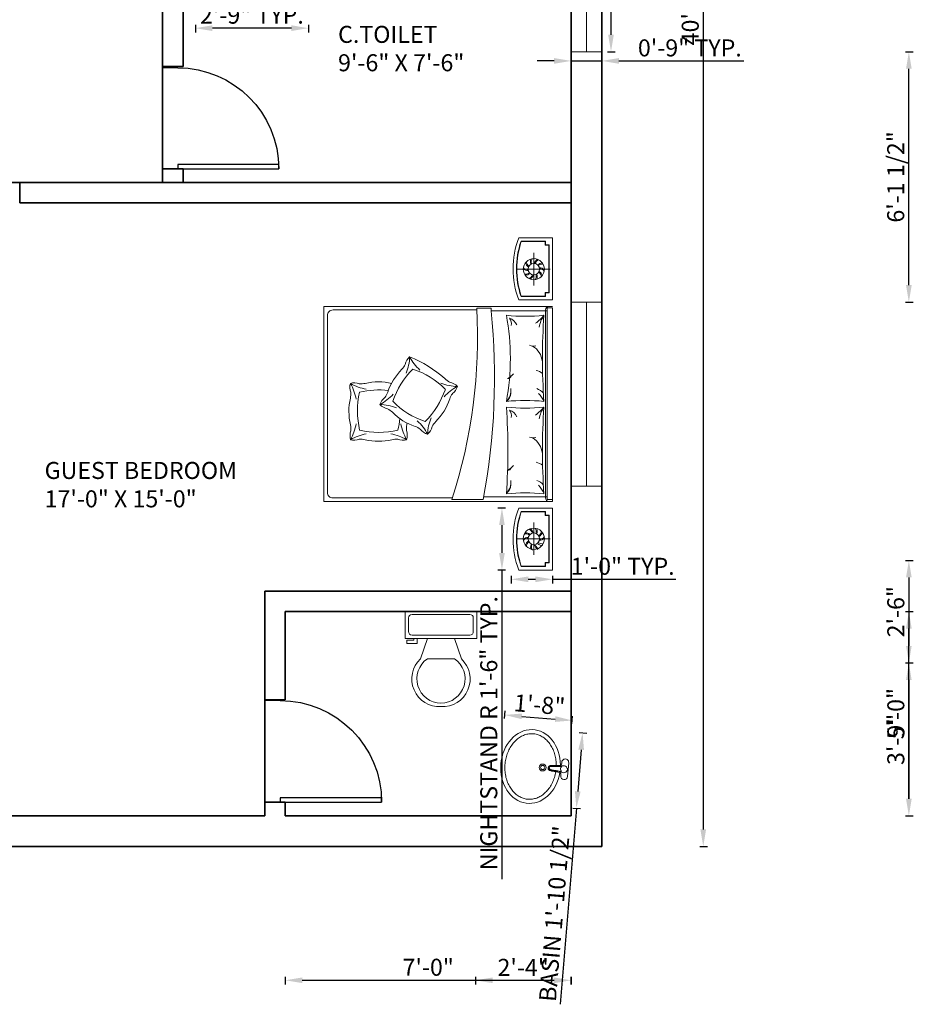
# Model space of a CAD drawing. Units: inches. Extents: x -48 to 817, y -530 to 78.
# Tile 5 of 7: x 551 to 817, y -515 to -225. Entities that reach past the tile are written whole.
import ezdxf

# ---------------------------------------------------------------- set-up
doc = ezdxf.new("R2010")
doc.units = ezdxf.units.IN
for name, color, linetype, lineweight in [('A-ANNO-DIMS', 2, 'Continuous', 18), ('A-AREA-IDEN', 7, 'Continuous', 18), ('A-DOOR', 3, 'Continuous', 25), ('A-FLOR-FIXT', 9, 'Continuous', 18), ('A-GLAZ', 4, 'Continuous', 18), ('A-WALL', 7, 'Continuous', 35), ('furn', 8, 'Continuous', 18)]:
    doc.layers.add(name, color=color, linetype=linetype, lineweight=lineweight)
doc.styles.get("Standard").update_dxf_attribs({"font": 'arial.ttf'})
doc.dimstyles.new('ISO-25', dxfattribs={"dimtxt": 5, "dimasz": 5, "dimexe": 1.25, "dimexo": 0.625, "dimtad": 1, "dimlunit": 3, "dimtxsty": 'Standard', "dimcen": 2.5, "dimadec": 0, "dimazin": 0, "dimtfac": 1, "dimtmove": 0, "dimatfit": 3, "dimfxl": 1, "dimfxlon": 1, "dimarcsym": 0})

# ---------------------------------------------------------------- blocks, each defined once
blk = doc.blocks.new('*U4')
for p, q in [((9.5, -6), (9.5, -2)), ((-10, -8.5), (-8, -8.5)), ((-10, -9.5), (-10, -8.5)), ((-8, -8.5), (-8, -8)), ((-7, -8), (-7, -9.5)), ((-4, -8), (-6, -14)), ((4, -8), (6, -14)), ((-7, -9.5), (-10, -9.5)), ((4, -14), (-4, -14))]:
    blk.add_line(p, q)
blk.add_lwpolyline([(10.5, -8), (10.5, 0), (-10.5, 0), (-10.5, -8)], close=True)
for points in [[(-9.5, -2), (-9.5, -6)], [(8.5, -1), (-8.5, -1)], [(-8.5, -7), (8.5, -7)]]:
    blk.add_lwpolyline(points)
for centre, radius, start, end in [((-8.625, -1.875), 0.8839, 81.8699, 188.1301), ((8.625, -1.875), 0.8839, 351.8699, 98.1301), ((-8.625, -6.125), 0.8839, 171.869898, 278.1301), ((8.625, -6.125), 0.8839, 261.8699, 8.1301), ((-0.4772, -19.9188), 8.0953, 133.01722, 273.38), ((0.0374, -19.8731), 7.127, 124.50543, 269.7), ((-0.0373, -19.8731), 7.127, 270.3, 55.4946), ((0.4773, -19.9188), 8.0953, 266.62, 46.9828)]:
    blk.add_arc(centre, radius, start, end)
blk = doc.blocks.new('*U2')
for p, q in [((0, 0), (0, -6)), ((40, 0), (40, -6))]:
    blk.add_line(p, q)
blk.add_lwpolyline([(0, 0), (0, 40), (1.75, 40), (1.75, 0)], close=True)
blk.add_arc((0, 0), 40, 0, 90)
blk = doc.blocks.new('A$C359865C9')
for p, q in [((0.26, 0.5858), (0.38, 0.5858)), ((0.26, 0.5258), (0.272, 0.5258)), ((0.368, 0.5258), (0.3809, 0.5258))]:
    blk.add_line(p, q)
for radius in [0.03, 0.018]:
    blk.add_circle((0.3201, 0.3632), radius)
for centre, radius, start, end in [((0.26, 0.5558), 0.03, 90.00613, 270.00613), ((0.272, 0.5078), 0.018, 0.00613, 90.00613), ((0.32, 0.5495), 0.03, 348.15369, 191.84631), ((0.32, 0.5495), 0.03, 222.45226, 317.54774), ((0.368, 0.5078), 0.018, 90.00613, 180.00613), ((0.38, 0.5558), 0.03, 270.00613, 89.98161), ((0.3201, 0.4358), 0.024, 180.00613, 0.00613), ((0.3201, 0.4358), 0.0204, 180.00613, 0.00613), ((0.3201, 0.4358), 0.0144, 180.00613, 0.00613)]:
    blk.add_arc(centre, radius, start, end)
at = {"ltscale": 100, "extrusion": (0, 0, -1)}
blk.add_ellipse((0.3201, 0.258), major_axis=(0.3216, 0), ratio=0.80597, start_param=-1.471508, end_param=4.612925, dxfattribs=at)
at = {"extrusion": (0, 0, -1)}
blk.add_ellipse((0.3199, 0.5826), major_axis=(-0.00812, 0), ratio=0.392595, dxfattribs=at)
for points, knots in [([(0.2907, 0.5434), (0.2946, 0.498), (0.2952, 0.4908), (0.2965, 0.4761), (0.2971, 0.4686), (0.2983, 0.4536), (0.2989, 0.4461), (0.2995, 0.4378), (0.2996, 0.4369), (0.2996, 0.4361)], [2.511178, 2.511178, 2.511178, 2.511178, 20.495008, 20.495008, 39.297594, 39.297594, 58.10018, 58.10018, 60.208758, 60.208758, 60.208758, 60.208758]), ([(0.2979, 0.5293), (0.298, 0.528), (0.2981, 0.5267), (0.2988, 0.5184), (0.2993, 0.5127), (0.3005, 0.4986), (0.301, 0.4933), (0.3014, 0.4884), (0.3015, 0.4875), (0.3017, 0.4857), (0.3017, 0.485), (0.3019, 0.4827), (0.3021, 0.4812), (0.3026, 0.4756), (0.3029, 0.4716), (0.3037, 0.4621), (0.3041, 0.4568), (0.3049, 0.4464), (0.3053, 0.4415), (0.3056, 0.4365)], [4.643985, 4.643985, 4.643985, 4.643985, 5.282102, 5.282102, 8.976667, 8.976667, 16.365798, 16.365798, 18.536065, 18.536065, 20.434607, 20.434607, 24.231692, 24.231692, 34.371999, 34.371999, 47.807513, 47.807513, 60.208758, 60.208758, 60.208758, 60.208758]), ([(0.3422, 0.5293), (0.3421, 0.528), (0.342, 0.5267), (0.3412, 0.5184), (0.3408, 0.5127), (0.3395, 0.4986), (0.3391, 0.4933), (0.3387, 0.4884), (0.3386, 0.4875), (0.3384, 0.4857), (0.3383, 0.485), (0.3381, 0.4827), (0.338, 0.4812), (0.3375, 0.4756), (0.3372, 0.4716), (0.3364, 0.4621), (0.336, 0.4568), (0.3352, 0.4464), (0.3348, 0.4415), (0.3345, 0.4365)], [4.643985, 4.643985, 4.643985, 4.643985, 5.282102, 5.282102, 8.976667, 8.976667, 16.365798, 16.365798, 18.536065, 18.536065, 20.434607, 20.434607, 24.231692, 24.231692, 34.371999, 34.371999, 47.807513, 47.807513, 60.208758, 60.208758, 60.208758, 60.208758]), ([(0.3494, 0.5434), (0.3455, 0.498), (0.3449, 0.4908), (0.3436, 0.4761), (0.343, 0.4686), (0.3418, 0.4536), (0.3412, 0.4461), (0.3406, 0.4378), (0.3405, 0.4369), (0.3404, 0.4361)], [2.511178, 2.511178, 2.511178, 2.511178, 20.495008, 20.495008, 39.297594, 39.297594, 58.10018, 58.10018, 60.208758, 60.208758, 60.208758, 60.208758]), ([(0.3475, 0.4801), (0.3477, 0.4801), (0.3479, 0.4801), (0.3648, 0.4788), (0.3813, 0.4763), (0.4136, 0.4692), (0.4293, 0.4645), (0.4593, 0.4531), (0.4737, 0.4464), (0.5006, 0.4312), (0.5131, 0.4227), (0.5361, 0.4042), (0.5465, 0.3942), (0.5649, 0.3732), (0.5729, 0.3622), (0.5864, 0.3393), (0.5918, 0.3275), (0.6, 0.3036), (0.6029, 0.2914), (0.6059, 0.2669), (0.6061, 0.2545), (0.6039, 0.2301), (0.6015, 0.218), (0.5941, 0.1942), (0.5892, 0.1825), (0.5768, 0.1597), (0.5693, 0.1486), (0.552, 0.1275), (0.5422, 0.1174), (0.5203, 0.0986), (0.5083, 0.0899), (0.4825, 0.0741), (0.4686, 0.0671), (0.4396, 0.0549), (0.4243, 0.0498), (0.3929, 0.0418), (0.3767, 0.0388), (0.3439, 0.0352), (0.3273, 0.0344), (0.2942, 0.0353), (0.2776, 0.0369), (0.2452, 0.0422), (0.2293, 0.046), (0.1987, 0.0556), (0.1839, 0.0615), (0.156, 0.0751), (0.1428, 0.0828), (0.1184, 0.0997), (0.1071, 0.109), (0.0869, 0.1288), (0.078, 0.1393), (0.0625, 0.1611), (0.0559, 0.1725), (0.0454, 0.1957), (0.0415, 0.2076), (0.036, 0.2317), (0.0346, 0.2438), (0.0345, 0.2566), (0.0345, 0.2573), (0.0345, 0.258), (0.0345, 0.2664), (0.0351, 0.2749), (0.0382, 0.2956), (0.0413, 0.3078), (0.0502, 0.3317), (0.0559, 0.3434), (0.0699, 0.3661), (0.0782, 0.377), (0.0972, 0.3978), (0.1079, 0.4076), (0.1313, 0.4257), (0.1441, 0.434), (0.1714, 0.4488), (0.186, 0.4553), (0.2163, 0.4662), (0.2321, 0.4706), (0.2628, 0.4769), (0.2776, 0.479), (0.2925, 0.4801)], [1.664851, 1.664851, 1.664851, 1.664851, 1.666804, 1.666804, 1.838807, 1.838807, 2.01081, 2.01081, 2.182814, 2.182814, 2.354817, 2.354817, 2.52682, 2.52682, 2.698824, 2.698824, 2.870827, 2.870827, 3.04283, 3.04283, 3.214834, 3.214834, 3.384783, 3.384783, 3.554732, 3.554732, 3.724681, 3.724681, 3.89463, 3.89463, 4.064578, 4.064578, 4.234527, 4.234527, 4.404476, 4.404476, 4.574425, 4.574425, 4.744374, 4.744374, 4.914323, 4.914323, 5.084272, 5.084272, 5.254221, 5.254221, 5.42417, 5.42417, 5.594119, 5.594119, 5.764068, 5.764068, 5.934016, 5.934016, 6.103965, 6.103965, 6.273914, 6.273914, 6.283185, 6.283185, 6.283185, 6.401959, 6.401959, 6.573962, 6.573962, 6.745965, 6.745965, 6.917969, 6.917969, 7.089972, 7.089972, 7.261975, 7.261975, 7.433979, 7.433979, 7.605982, 7.605982, 7.759676, 7.759676, 7.759676, 7.759676]), ([(0.29, 0.5078), (0.2913, 0.4937), (0.2935, 0.4697), (0.2953, 0.4457), (0.2961, 0.4358)], [0, 0, 0, 0, 35.358253, 60.208758, 60.208758, 60.208758, 60.208758]), ([(0.35, 0.5078), (0.3487, 0.4937), (0.3466, 0.4697), (0.3448, 0.4457), (0.344, 0.4358)], [0, 0, 0, 0, 35.358253, 60.208758, 60.208758, 60.208758, 60.208758])]:
    blk.add_open_spline(points, degree=3, knots=knots)
blk = doc.blocks.new('*D10')
at = {"layer": 'A-ANNO-DIMS', "color": 0, "lineweight": -2, "transparency": 16777216}
for p, q in [((751.22, 11.72), (753.47, 11.72)), ((752.22, 6.72), (752.22, -463.28)), ((751.22, -468.28), (753.47, -468.28))]:
    blk.add_line(p, q, dxfattribs=at)
at = {"layer": 'A-ANNO-DIMS', "color": 0, "transparency": 16777216}
for points in [[(751.39, 6.72), (753.06, 6.72), (752.22, 11.72)], [(751.39, -463.28), (753.06, -463.28), (752.22, -468.28)]]:
    blk.add_solid(points, dxfattribs=at)
at = {"layer": 'Defpoints', "color": 0, "transparency": 16777216}
for p in [(729.44, 11.72), (722.43, -468.28), (752.22, -468.28)]:
    blk.add_point(p, dxfattribs=at)
at = {"layer": 'A-ANNO-DIMS', "color": 0, "transparency": 16777216, "insert": (749.05, -228.28), "char_height": 5, "attachment_point": 5, "rotation": 90}
blk.add_mtext("40'", dxfattribs=at)
blk = doc.blocks.new('BED-DOUBLE')
for p, q in [((0.99, 65.08), (56.21, 65.08)), ((1.28, 65.57), (1.28, 49.06)), ((55.89, 65.57), (55.89, 46.91))]:
    blk.add_line(p, q)
for points in [[(0, 67.12), (0, 0), (57.2, 0), (57.2, 67.12)], [(56.67, 67.12), (56.67, 65.57), (0.33, 65.57), (0.33, 67.12), (57.2, 67.12)]]:
    blk.add_lwpolyline(points)
for points in [[(2.54, 53.57, 0.058596), (2.54, 64.62, 0.036889), (27.85, 64.62, 0.052163), (27.85, 53.57, 0.093111)], [(29.5, 53.57, 0.058596), (29.5, 64.62, 0.036648), (54.99, 64.62, 0.052163), (54.99, 53.57, 0.036967)], [(0.5, 49.06), (1.28, 49.06, -0.072944), (56.67, 46.75), (56.67, 37.58, 0.092568), (0.5, 44.85)]]:
    blk.add_lwpolyline(points, format="xyb", close=True)
for points in [[(0.99, 44.88), (0.99, 2.65, 0.414214), (2.65, 0.99), (54.56, 0.99, 0.414214), (56.21, 2.65), (56.21, 37.74)], [(22.46, 34.35, 0.091296), (23.47, 39.19, 0.091296), (26.52, 35.29, 0.091296)], [(18.37, 26.07, 0.111006), (27.81, 20.2, 0.119549), (33.77, 29.75, 0.107813), (24.35, 35.65)], [(24.3, 35.64, 0.121865), (18.37, 26.07, 0.121865)], [(28.76, 16.41, 0.159461), (30.04, 18.69, -0.076283), (31.05, 20.1, 0.115075), (35.2, 26.76, -0.076283), (36.02, 28.3, 0.159461), (37.5, 30.45)], [(32.66, 31.47, 0.091296), (37.5, 30.45, 0.091296), (33.59, 27.41, 0.091296)], [(19.57, 24.14, 0.091296), (14.72, 25.16, 0.091296), (18.63, 28.19, 0.091296)], [(34.44, 22.59, 0.091296), (39.09, 24.28, 0.091296), (37.38, 19.64, 0.091296)], [(39.09, 7.75, 0.159461), (38.98, 10.35, -0.076283), (39.09, 12.09, 0.115075), (39.09, 19.94, -0.076283), (38.98, 21.68, 0.159461), (39.09, 24.28)], [(25.17, 10.45, 0.111006), (36.29, 10.46, 0.119549), (36.29, 21.72, 0.033212), (32.87, 22.24)], [(29.76, 21.26, 0.091296), (28.76, 16.41, 0.091296), (25.71, 20.31)], [(27.21, 9.44, 0.091296), (22.56, 7.75, 0.091296), (24.27, 12.39, 0.091296)], [(37.38, 12.39, 0.091296), (39.09, 7.75, 0.091296), (34.44, 9.44)]]:
    blk.add_lwpolyline(points, format="xyb")
for centre, radius, start, end in [((0.99, 66.07), 0.992, 180, 270), ((8.41, 73.86), 10.95, 237.5379, 257.5233), ((-5.75, 54.29), 13.24, 36.4935, 51.2792), ((16.81, 58.07), 6.13, 96.6849, 148.3182), ((23.01, 61.56), 4.3, 141.8174, 169.8987), ((28.45, 60.95), 4.63, 130.5354, 160.3558), ((31.33, 57.05), 8.33, 114.6457, 134.1585), ((21.22, 54.29), 13.24, 36.4935, 51.2792), ((35.38, 73.86), 10.95, 237.5379, 257.5233), ((43.78, 58.07), 6.13, 96.6849, 148.3182), ((49.97, 61.56), 4.3, 141.8174, 169.8987), ((55.41, 60.95), 4.63, 130.5354, 160.3558), ((58.29, 57.05), 8.33, 114.6457, 134.1585), ((56.21, 66.07), 0.992, 270, 0), ((8.86, 61.48), 2.75, 335.8927, 16.1192), ((35.82, 61.48), 2.75, 335.8927, 16.1192), ((6.89, 53.32), 3.67, 114.2916, 160.9896), ((4.98, 52.55), 2.51, 76.4823, 128.5563), ((9.99, 45.89), 13.8, 36.2085, 45.0849), ((20.2, 54.04), 0.927, 353.7543, 77.2187), ((33.85, 53.32), 3.67, 114.2916, 160.9896), ((31.95, 52.55), 2.51, 76.4823, 128.5563), ((36.95, 45.89), 13.8, 36.2085, 45.0849), ((47.16, 54.04), 0.927, 353.7543, 77.2187), ((24.63, 50.41), 4.52, 44.406, 96.8342), ((25.47, 51.99), 2.86, 33.6349, 90.8456), ((51.59, 50.41), 4.52, 44.406, 96.8342), ((52.44, 51.99), 2.86, 33.6349, 90.8456), ((26.3, 36.1), 4.19, 132.4658, 168.7065), ((22.36, 35.3), 4.04, 37.2937, 74.0973), ((29.01, 42.35), 5.74, 233.2983, 250.7472), ((48.24, 11.46), 36.21, 138.3818, 157.7644), ((17.07, 39.52), 5.74, 315.5854, 333.0343), ((21.6, 20.56), 17.28, 45.1307, 71.3884), ((37.79, 36.92), 5.74, 225.7718, 243.2208), ((34.51, 27.99), 3.87, 39.4726, 79.6505), ((17.81, 28), 4.19, 222.6522, 258.8929), ((14.41, 18.76), 5.74, 45.7718, 63.2208), ((30.83, 7.48), 17.28, 77.0576, 78.7033), ((35.92, 29.93), 5.74, 257.6988, 275.1477), ((37.86, 20.61), 3.87, 71.3996, 111.5774), ((30.61, 35.12), 17.28, 225.1307, 251.3884), ((39.38, 16.01), 17.28, 166.8711, 193.1289), ((47.91, 16.13), 23.44, 173.1956, 194.0284), ((23.2, 13.33), 5.74, 53.2983, 70.7472), ((30.37, 20.93), 4.79, 218.7754, 250.3571), ((16.95, 10.85), 5.74, 355.0387, 12.4877), ((26.6, 8.88), 4.19, 159.3666, 195.6073), ((23.67, 11.79), 4.19, 254.5791, 290.8198), ((25.68, 2.15), 5.74, 77.6988, 95.1477), ((30.77, 24.6), 17.28, 257.0576, 283.3153), ((36.01, 2.19), 5.74, 85.2252, 102.6741), ((38.07, 12.43), 4.79, 250.7023, 282.284)]:
    blk.add_arc(centre, radius, start, end)
blk = doc.blocks.new('NIGHTSTAND-WITH-LAMP-L')
for p, q in [((9.19, 1.33), (9.19, 10.86)), ((4.42, 6.1), (13.95, 6.1))]:
    blk.add_line(p, q)
blk.add_lwpolyline([(0, 1.65), (0, 11.57), (18.19, 11.57), (18.19, 1.65, -0.181818)], format="xyb", close=True)
for points in [[(2.08, 10.58), (2.08, 9.49), (0.99, 9.49)], [(2.18, 10.58), (2.18, 9.39), (0.99, 9.39)], [(2.08, 10.58), (16.1, 10.58)], [(2.08, 10.48), (16.1, 10.48)], [(16, 10.58), (16, 9.39), (17.19, 9.39)], [(16.1, 10.58), (16.1, 9.49), (17.19, 9.49)]]:
    blk.add_lwpolyline(points)
for points in [[(17.19, 9.49), (17.19, 2.35, -0.167087), (0.99, 2.35), (0.99, 9.49)], [(17.09, 9.49), (17.09, 2.42, -0.165559), (1.09, 2.42), (1.09, 9.49)]]:
    blk.add_lwpolyline(points, format="xyb")
for radius in [3.11, 1.69]:
    blk.add_circle((9.19, 6.1), radius)
for centre, radius, start, end in [((9.46, 8.43), 2, 172.17, 218.4897), ((9.27, 8.39), 1.53, 160.3002, 220.538), ((10.78, 7.82), 2, 136.17, 182.4897), ((10.6, 7.9), 1.53, 124.3002, 184.538), ((8.04, 8.15), 2, 208.17, 254.4897), ((7.91, 8), 1.53, 196.3002, 256.538), ((11.49, 6.56), 2, 100.17, 146.4897), ((11.39, 6.73), 1.53, 88.3002, 148.538), ((11.32, 5.11), 2, 64.17, 110.4897), ((11.34, 5.31), 1.53, 52.3002, 112.538), ((10.33, 4.05), 2, 28.17, 74.4897), ((7.03, 6.88), 1.53, 232.3002, 292.538), ((7.05, 7.08), 2, 244.17, 290.4897), ((6.98, 5.47), 1.53, 268.3002, 328.538), ((6.88, 5.64), 2, 280.17, 326.4897), ((7.78, 4.29), 1.53, 304.3002, 4.538), ((7.59, 4.37), 2, 316.17, 2.4897), ((9.11, 3.81), 1.53, 340.3002, 40.538), ((8.91, 3.76), 2, 352.17, 38.4897), ((10.47, 4.2), 1.53, 16.3002, 76.538)]:
    blk.add_arc(centre, radius, start, end)
blk = doc.blocks.new('NIGHTSTAND-WITH-LAMP-R')
for p, q in [((9, 1.32), (9, 10.86)), ((13.77, 6.09), (4.23, 6.09))]:
    blk.add_line(p, q)
blk.add_lwpolyline([(18.19, 1.65), (18.19, 11.57), (0, 11.57), (0, 1.65, 0.181818)], format="xyb", close=True)
for points in [[(2.08, 10.58), (2.08, 9.49), (0.99, 9.49)], [(2.18, 10.58), (2.18, 9.39), (0.99, 9.39)], [(16.1, 10.58), (2.08, 10.58)], [(16.1, 10.48), (2.08, 10.48)], [(16, 10.58), (16, 9.39), (17.19, 9.39)], [(16.1, 10.58), (16.1, 9.49), (17.19, 9.49)]]:
    blk.add_lwpolyline(points)
for points in [[(0.99, 9.49), (0.99, 2.35, 0.167087), (17.19, 2.35), (17.19, 9.49)], [(1.09, 9.49), (1.09, 2.42, 0.165559), (17.09, 2.42), (17.09, 9.49)]]:
    blk.add_lwpolyline(points, format="xyb")
for radius in [3.11, 1.69]:
    blk.add_circle((9, 6.09), radius)
for centre, radius, start, end in [((7.59, 7.9), 1.53, 355.462, 55.6998), ((7.4, 7.82), 2, 357.5103, 43.83), ((8.92, 8.38), 1.53, 319.462, 19.6998), ((8.95, 8.51), 2, 321.5103, 7.83), ((6.85, 5.31), 1.53, 67.462, 127.6998), ((6.87, 5.11), 2, 69.5103, 115.83), ((7.85, 4.04), 2, 105.5103, 151.83), ((6.8, 6.72), 1.53, 31.462, 91.6998), ((6.69, 6.55), 2, 33.5103, 79.83), ((10.51, 8.08), 1.53, 283.462, 343.6998), ((10.37, 8.23), 2, 285.5103, 331.83), ((7.72, 4.19), 1.53, 103.462, 163.6998), ((9.27, 3.76), 2, 141.5103, 187.83), ((9.08, 3.8), 1.53, 139.462, 199.6998), ((10.59, 4.37), 2, 177.5103, 223.83), ((10.41, 4.29), 1.53, 175.462, 235.6998), ((11.3, 5.63), 2, 213.5103, 259.83), ((11.2, 5.46), 1.53, 211.462, 271.6998), ((11.36, 7.16), 2, 249.5103, 295.83), ((11.38, 6.96), 1.53, 247.462, 307.6998)]:
    blk.add_arc(centre, radius, start, end)
blk = doc.blocks.new('WIN-54IN')
blk.add_line((4.5, 54), (4.5, 0))
blk.add_lwpolyline([(9, 54), (0, 54), (0, 0), (9, 0)], close=True)
blk = doc.blocks.new('WIN-18IN')
blk.add_line((4.5, 18), (4.5, 0))
blk.add_lwpolyline([(0, 18), (9, 18), (9, 0), (0, 0)], close=True)
blk = doc.blocks.new('*D24')
at = {"layer": 'A-ANNO-DIMS', "color": 0, "lineweight": -2, "transparency": 16777216}
for p, q in [((725.13, -216.89), (725.13, -147.37)), ((724.13, -216.89), (726.38, -216.89)), ((725.13, -229.89), (725.13, -221.89)), ((724.13, -234.89), (726.38, -234.89))]:
    blk.add_line(p, q, dxfattribs=at)
at = {"layer": 'A-ANNO-DIMS', "color": 0, "transparency": 16777216}
for points in [[(724.29, -221.89), (725.96, -221.89), (725.13, -216.89)], [(724.29, -229.89), (725.96, -229.89), (725.13, -234.89)]]:
    blk.add_solid(points, dxfattribs=at)
at = {"layer": 'Defpoints', "color": 0, "transparency": 16777216}
for p in [(722.43, -216.89), (725.13, -216.89), (722.43, -234.89)]:
    blk.add_point(p, dxfattribs=at)
at = {"layer": 'A-ANNO-DIMS', "color": 0, "transparency": 16777216, "insert": (721.92, -179.63), "char_height": 5, "attachment_point": 5, "rotation": 90}
blk.add_mtext('WINDOW 1\'-6" TYP.', dxfattribs=at)
blk = doc.blocks.new('*D25')
at = {"layer": 'A-ANNO-DIMS', "color": 0, "lineweight": -2, "transparency": 16777216}
for p, q in [((713.43, -236.59), (713.43, -238.84)), ((722.43, -236.59), (722.43, -238.84)), ((708.43, -237.59), (703.43, -237.59)), ((713.43, -237.59), (722.43, -237.59)), ((727.43, -237.59), (764.15, -237.59))]:
    blk.add_line(p, q, dxfattribs=at)
at = {"layer": 'A-ANNO-DIMS', "color": 0, "transparency": 16777216}
for points in [[(708.43, -236.75), (708.43, -238.42), (713.43, -237.59)], [(727.43, -236.75), (727.43, -238.42), (722.43, -237.59)]]:
    blk.add_solid(points, dxfattribs=at)
at = {"layer": 'Defpoints', "color": 0, "transparency": 16777216}
for p in [(713.43, -234.89), (722.43, -234.89), (722.43, -237.59)]:
    blk.add_point(p, dxfattribs=at)
at = {"layer": 'A-ANNO-DIMS', "color": 0, "transparency": 16777216, "insert": (748.29, -234.41), "char_height": 5, "attachment_point": 5}
blk.add_mtext('0\'-9" TYP.', dxfattribs=at)
blk = doc.blocks.new('*D29')
at = {"layer": 'A-ANNO-DIMS', "color": 0, "lineweight": -2, "transparency": 16777216}
for p, q in [((603.04, -226.97), (603.04, -229.22)), ((631.24, -227.97), (608.04, -227.97)), ((636.24, -226.97), (636.24, -229.22))]:
    blk.add_line(p, q, dxfattribs=at)
at = {"layer": 'A-ANNO-DIMS', "color": 0, "transparency": 16777216}
for points in [[(608.04, -227.13), (608.04, -228.8), (603.04, -227.97)], [(631.24, -227.13), (631.24, -228.8), (636.24, -227.97)]]:
    blk.add_solid(points, dxfattribs=at)
at = {"layer": 'Defpoints', "color": 0, "transparency": 16777216}
for p in [(603.04, -222.37), (636.24, -222.37), (603.04, -227.97)]:
    blk.add_point(p, dxfattribs=at)
at = {"layer": 'A-ANNO-DIMS', "color": 0, "transparency": 16777216, "insert": (619.64, -224.79), "char_height": 5, "attachment_point": 5}
blk.add_mtext('2\'-9" TYP.', dxfattribs=at)
blk = doc.blocks.new('*D30')
at = {"layer": 'A-ANNO-DIMS', "color": 0, "lineweight": -2, "transparency": 16777216}
for p, q in [((715.77, -434.81), (718.01, -434.99)), ((716.36, -439.87), (715.36, -452.1)), ((714.95, -457.08), (710.23, -514.64)), ((713.95, -457), (716.19, -457.18))]:
    blk.add_line(p, q, dxfattribs=at)
at = {"layer": 'A-ANNO-DIMS', "color": 0, "transparency": 16777216}
for points in [[(715.53, -439.81), (717.19, -439.94), (716.77, -434.89)], [(714.53, -452.03), (716.19, -452.17), (714.95, -457.08)]]:
    blk.add_solid(points, dxfattribs=at)
at = {"layer": 'Defpoints', "color": 0, "transparency": 16777216}
for p in [(713.44, -434.62), (711.62, -456.81), (714.95, -457.08)]:
    blk.add_point(p, dxfattribs=at)
at = {"layer": 'A-ANNO-DIMS', "color": 0, "transparency": 16777216, "insert": (709.19, -488.09), "char_height": 5, "attachment_point": 5, "rotation": 85.3161}
blk.add_mtext('BASIN 1\'-10 1/2"', dxfattribs=at)
blk = doc.blocks.new('*D31')
at = {"layer": 'A-ANNO-DIMS', "color": 0, "lineweight": -2, "transparency": 16777216}
for p, q in [((693.87, -430.67), (694.06, -428.42)), ((698.94, -430.08), (708.73, -430.88)), ((713.63, -432.29), (713.81, -430.04))]:
    blk.add_line(p, q, dxfattribs=at)
at = {"layer": 'A-ANNO-DIMS', "color": 0, "transparency": 16777216}
for points in [[(699.01, -429.25), (698.87, -430.91), (693.95, -429.67)], [(708.79, -430.05), (708.66, -431.71), (713.71, -431.29)]]:
    blk.add_solid(points, dxfattribs=at)
at = {"layer": 'Defpoints', "color": 0, "transparency": 16777216}
for p in [(693.68, -433), (713.71, -431.29), (713.44, -434.62)]:
    blk.add_point(p, dxfattribs=at)
at = {"layer": 'A-ANNO-DIMS', "color": 0, "transparency": 16777216, "insert": (704.09, -427.31), "char_height": 5, "attachment_point": 5, "rotation": 355.3161}
blk.add_mtext('1\'-8"', dxfattribs=at)
blk = doc.blocks.new('*D36')
at = {"layer": 'A-ANNO-DIMS', "color": 0, "lineweight": -2, "transparency": 16777216}
for p, q in [((694.09, -368.92), (691.84, -368.92)), ((693.09, -373.92), (693.09, -382.1)), ((694.09, -387.1), (691.84, -387.1)), ((693.09, -387.1), (693.09, -477.92))]:
    blk.add_line(p, q, dxfattribs=at)
at = {"layer": 'A-ANNO-DIMS', "color": 0, "transparency": 16777216}
for points in [[(692.25, -373.92), (693.92, -373.92), (693.09, -368.92)], [(692.25, -382.1), (693.92, -382.1), (693.09, -387.1)]]:
    blk.add_solid(points, dxfattribs=at)
at = {"layer": 'Defpoints', "color": 0, "transparency": 16777216}
for p in [(695.81, -368.92), (693.09, -387.1), (695.81, -387.1)]:
    blk.add_point(p, dxfattribs=at)
at = {"layer": 'A-ANNO-DIMS', "color": 0, "transparency": 16777216, "insert": (689.87, -435.01), "char_height": 5, "attachment_point": 5, "rotation": 90}
blk.add_mtext('NIGHTSTAND R 1\'-6" TYP.', dxfattribs=at)
blk = doc.blocks.new('*D37')
at = {"layer": 'A-ANNO-DIMS', "color": 0, "lineweight": -2, "transparency": 16777216}
for p, q in [((695.81, -388.83), (695.81, -391.08)), ((700.81, -389.83), (702.94, -389.83)), ((707.94, -388.83), (707.94, -391.08)), ((707.94, -389.83), (744.19, -389.83))]:
    blk.add_line(p, q, dxfattribs=at)
at = {"layer": 'A-ANNO-DIMS', "color": 0, "transparency": 16777216}
for points in [[(700.81, -389), (700.81, -390.67), (695.81, -389.83)], [(702.94, -389), (702.94, -390.67), (707.94, -389.83)]]:
    blk.add_solid(points, dxfattribs=at)
at = {"layer": 'Defpoints', "color": 0, "transparency": 16777216}
for p in [(695.81, -387.1), (707.94, -387.1), (707.94, -389.83)]:
    blk.add_point(p, dxfattribs=at)
at = {"layer": 'A-ANNO-DIMS', "color": 0, "transparency": 16777216, "insert": (728.56, -386.65), "char_height": 5, "attachment_point": 5}
blk.add_mtext('1\'-0" TYP.', dxfattribs=at)
blk = doc.blocks.new('*D42')
at = {"layer": 'A-ANNO-DIMS', "color": 0, "lineweight": -2, "transparency": 16777216}
for p, q in [((629.43, -506.59), (629.43, -508.84)), ((634.43, -507.59), (708.43, -507.59)), ((713.43, -506.59), (713.43, -508.84))]:
    blk.add_line(p, q, dxfattribs=at)
at = {"layer": 'A-ANNO-DIMS', "color": 0, "transparency": 16777216}
for points in [[(634.43, -506.76), (634.43, -508.42), (629.43, -507.59)], [(708.43, -506.76), (708.43, -508.42), (713.43, -507.59)]]:
    blk.add_solid(points, dxfattribs=at)
at = {"layer": 'Defpoints', "color": 0, "transparency": 16777216}
for p in [(629.43, -459.28), (713.43, -459.28), (713.43, -507.59)]:
    blk.add_point(p, dxfattribs=at)
at = {"layer": 'A-ANNO-DIMS', "color": 0, "transparency": 16777216, "insert": (671.43, -504.41), "char_height": 5, "attachment_point": 5}
blk.add_mtext('7\'-0"', dxfattribs=at)
blk = doc.blocks.new('*D43')
at = {"layer": 'A-ANNO-DIMS', "color": 0, "lineweight": -2, "transparency": 16777216}
for p, q in [((811.62, -399.28), (813.87, -399.28)), ((812.62, -454.28), (812.62, -404.28)), ((811.62, -459.28), (813.87, -459.28))]:
    blk.add_line(p, q, dxfattribs=at)
at = {"layer": 'A-ANNO-DIMS', "color": 0, "transparency": 16777216}
for points in [[(811.79, -404.28), (813.45, -404.28), (812.62, -399.28)], [(811.79, -454.28), (813.45, -454.28), (812.62, -459.28)]]:
    blk.add_solid(points, dxfattribs=at)
at = {"layer": 'Defpoints', "color": 0, "transparency": 16777216}
for p in [(713.43, -399.28), (812.62, -399.28), (713.43, -459.28)]:
    blk.add_point(p, dxfattribs=at)
at = {"layer": 'A-ANNO-DIMS', "color": 0, "transparency": 16777216, "insert": (809.44, -429.28), "char_height": 5, "attachment_point": 5, "rotation": 90}
blk.add_mtext('5\'-0"', dxfattribs=at)
blk = doc.blocks.new('*D55')
at = {"layer": 'A-ANNO-DIMS', "color": 0, "lineweight": -2, "transparency": 16777216}
for p, q in [((811.62, -234.89), (813.87, -234.89)), ((812.62, -303.44), (812.62, -239.89)), ((811.62, -308.44), (813.87, -308.44))]:
    blk.add_line(p, q, dxfattribs=at)
at = {"layer": 'A-ANNO-DIMS', "color": 0, "transparency": 16777216}
for points in [[(811.79, -239.89), (813.45, -239.89), (812.62, -234.89)], [(811.79, -303.44), (813.45, -303.44), (812.62, -308.44)]]:
    blk.add_solid(points, dxfattribs=at)
at = {"layer": 'Defpoints', "color": 0, "transparency": 16777216}
for p in [(722.43, -234.89), (812.62, -234.89), (722.43, -308.44)]:
    blk.add_point(p, dxfattribs=at)
at = {"layer": 'A-ANNO-DIMS', "color": 0, "transparency": 16777216, "insert": (809.41, -271.66), "char_height": 5, "attachment_point": 5, "rotation": 90}
blk.add_mtext('6\'-1 1/2"', dxfattribs=at)
blk = doc.blocks.new('*D62')
at = {"layer": 'A-ANNO-DIMS', "color": 0, "lineweight": -2, "transparency": 16777216}
for p, q in [((-35.87, -239.28), (-38.12, -239.28)), ((-36.87, -244.28), (-36.87, -264.28)), ((-35.87, -269.28), (-38.12, -269.28))]:
    blk.add_line(p, q, dxfattribs=at)
at = {"layer": 'A-ANNO-DIMS', "color": 0, "transparency": 16777216}
for points in [[(-37.71, -244.28), (-36.04, -244.28), (-36.87, -239.28)], [(-37.71, -264.28), (-36.04, -264.28), (-36.87, -269.28)]]:
    blk.add_solid(points, dxfattribs=at)
at = {"layer": 'Defpoints', "color": 0, "transparency": 16777216}
for p in [(593.43, -239.28), (-36.87, -269.28), (593.43, -269.28)]:
    blk.add_point(p, dxfattribs=at)
at = {"layer": 'A-ANNO-DIMS', "color": 0, "transparency": 16777216, "insert": (-40.05, -254.28), "char_height": 5, "attachment_point": 5, "rotation": 90}
blk.add_mtext('2\'-6"', dxfattribs=at)
blk = doc.blocks.new('*D65')
at = {"layer": 'A-ANNO-DIMS', "color": 0, "lineweight": -2, "transparency": 16777216}
for p, q in [((811.62, -384.28), (813.87, -384.28)), ((812.62, -389.28), (812.62, -409.4)), ((811.62, -414.4), (813.87, -414.4))]:
    blk.add_line(p, q, dxfattribs=at)
at = {"layer": 'A-ANNO-DIMS', "color": 0, "transparency": 16777216}
for points in [[(811.79, -389.28), (813.45, -389.28), (812.62, -384.28)], [(811.79, -409.4), (813.45, -409.4), (812.62, -414.4)]]:
    blk.add_solid(points, dxfattribs=at)
at = {"layer": 'Defpoints', "color": 0, "transparency": 16777216}
for p in [(161.43, -384.28), (161.43, -414.4), (812.62, -414.4)]:
    blk.add_point(p, dxfattribs=at)
at = {"layer": 'A-ANNO-DIMS', "color": 0, "transparency": 16777216, "insert": (809.44, -399.34), "char_height": 5, "attachment_point": 5, "rotation": 90}
blk.add_mtext('2\'-6"', dxfattribs=at)
blk = doc.blocks.new('*D66')
at = {"layer": 'A-ANNO-DIMS', "color": 0, "lineweight": -2, "transparency": 16777216}
for p, q in [((811.62, -414.4), (813.87, -414.4)), ((812.62, -419.4), (812.62, -454.28)), ((811.62, -459.28), (813.87, -459.28))]:
    blk.add_line(p, q, dxfattribs=at)
at = {"layer": 'A-ANNO-DIMS', "color": 0, "transparency": 16777216}
for points in [[(811.79, -419.4), (813.45, -419.4), (812.62, -414.4)], [(811.79, -454.28), (813.45, -454.28), (812.62, -459.28)]]:
    blk.add_solid(points, dxfattribs=at)
at = {"layer": 'Defpoints', "color": 0, "transparency": 16777216}
for p in [(161.43, -414.4), (161.43, -459.28), (812.62, -459.28)]:
    blk.add_point(p, dxfattribs=at)
at = {"layer": 'A-ANNO-DIMS', "color": 0, "transparency": 16777216, "insert": (809.44, -436.84), "char_height": 5, "attachment_point": 5, "rotation": 90}
blk.add_mtext('3\'-9"', dxfattribs=at)
blk = doc.blocks.new('*D81')
at = {"layer": 'A-ANNO-DIMS', "color": 0, "lineweight": -2, "transparency": 16777216}
for p, q in [((685.32, -506.59), (685.32, -508.84)), ((690.32, -507.59), (708.32, -507.59)), ((713.32, -506.59), (713.32, -508.84))]:
    blk.add_line(p, q, dxfattribs=at)
at = {"layer": 'A-ANNO-DIMS', "color": 0, "transparency": 16777216}
for points in [[(690.32, -506.76), (690.32, -508.42), (685.32, -507.59)], [(708.32, -506.76), (708.32, -508.42), (713.32, -507.59)]]:
    blk.add_solid(points, dxfattribs=at)
at = {"layer": 'Defpoints', "color": 0, "transparency": 16777216}
for p in [(685.32, -47.75), (713.32, -58.25), (713.32, -507.59)]:
    blk.add_point(p, dxfattribs=at)
at = {"layer": 'A-ANNO-DIMS', "color": 0, "transparency": 16777216, "insert": (699.32, -504.45), "char_height": 5, "attachment_point": 5}
blk.add_mtext('2\'-4"', dxfattribs=at)
blk = doc.blocks.new('*D84')
at = {"layer": 'A-ANNO-DIMS', "color": 0, "lineweight": -2, "transparency": 16777216}
for p, q in [((-35.87, -425.28), (-38.12, -425.28)), ((-36.87, -450.28), (-36.87, -430.28)), ((-35.87, -455.28), (-38.12, -455.28))]:
    blk.add_line(p, q, dxfattribs=at)
at = {"layer": 'A-ANNO-DIMS', "color": 0, "transparency": 16777216}
for points in [[(-37.71, -430.28), (-36.04, -430.28), (-36.87, -425.28)], [(-37.71, -450.28), (-36.04, -450.28), (-36.87, -455.28)]]:
    blk.add_solid(points, dxfattribs=at)
at = {"layer": 'Defpoints', "color": 0, "transparency": 16777216}
for p in [(-36.87, -425.28), (623.43, -425.28), (623.43, -455.28)]:
    blk.add_point(p, dxfattribs=at)
at = {"layer": 'A-ANNO-DIMS', "color": 0, "transparency": 16777216, "insert": (-40.05, -440.28), "char_height": 5, "attachment_point": 5, "rotation": 90}
blk.add_mtext('2\'-6"', dxfattribs=at)

msp = doc.modelspace()

# ---------------------------------------------------------------- linework, layer by layer
at = {"layer": 'A-WALL'}
for p, q in [((722.427, 11.725), (722.427, -468.275)), ((713.427, 2.725), (713.427, -459.275)), ((593.427, -183.275), (593.427, -273.275)), ((599.427, -183.275), (599.427, -239.275)), ((599.427, -239.275), (593.427, -239.275)), ((599.427, -269.275), (593.427, -269.275)), ((599.427, -269.275), (599.427, -273.275)), ((509.427, -273.275), (713.427, -273.275)), ((551.427, -279.275), (551.427, -273.275)), ((551.427, -279.275), (713.427, -279.275)), ((713.427, -393.275), (623.427, -393.275)), ((623.427, -399.275), (623.427, -393.275)), ((623.427, -399.275), (623.427, -459.275)), ((713.427, -399.275), (629.427, -399.275)), ((629.427, -399.275), (629.427, -425.275)), ((629.427, -425.275), (623.427, -425.275)), ((629.427, -455.275), (623.427, -455.275)), ((629.427, -455.275), (629.427, -459.275)), ((623.427, -459.275), (308.498, -459.275)), ((713.427, -459.275), (629.427, -459.275)), ((722.427, -468.275), (2.427, -468.275))]:
    msp.add_line(p, q, dxfattribs=at)

# ---------------------------------------------------------------- block references
at = {"layer": 'A-DOOR', "rotation": 270}
for p, xscale, yscale, zscale in [((597.877, -269.275), -0.7416502636543669, 0.7416502636543669, 0.7416502636543669), ((627.904, -455.275), -0.7460762736299266, 0.7460762736299266, 0.7460762736299266)]:
    msp.add_blockref('*U2', p, dxfattribs=dict(at, xscale=xscale, yscale=yscale, zscale=zscale))
at = {"layer": 'A-FLOR-FIXT'}
msp.add_blockref('*U4', (675.176, -399.191), dxfattribs=at)
at = {"layer": 'A-FLOR-FIXT', "xscale": 33.76335769858793, "yscale": 33.76335769858793, "zscale": 33.76335769858793, "rotation": 265.3160831367992}
msp.add_blockref('A$C359865C9', (693.698, -433.327), dxfattribs=at)
at = {"layer": 'A-GLAZ'}
for name, p in [('WIN-18IN', (713.427, -234.886)), ('WIN-54IN', (713.427, -362.439))]:
    msp.add_blockref(name, p, dxfattribs=at)
at = {"layer": 'furn'}
for name, p, rotation in [('NIGHTSTAND-WITH-LAMP-L', (696.36, -289.565), 270.0000000000021), ('BED-DOUBLE', (640.816, -309.734), 270), ('NIGHTSTAND-WITH-LAMP-R', (696.363, -368.92), 270.0000000000001)]:
    msp.add_blockref(name, p, dxfattribs=dict(at, rotation=rotation))

# ---------------------------------------------------------------- texts
at = {"layer": 'A-AREA-IDEN', "char_height": 5, "attachment_point": 1}
for s, width, insert in [('C.TOILET\\P9\'-6" X 7\'-6"', 50.63289, (644.946, -227.293)), ('GUEST BEDROOM\\P17\'-0" X 15\'-0"', 64.6775, (558.75, -355.363))]:
    msp.add_mtext_dynamic_manual_height_columns(s, width=width, gutter_width=12.5, heights=[0], dxfattribs=dict(at, insert=insert))

# ---------------------------------------------------------------- dimensions: what is measured, and where the dimension line sits
at = {"layer": 'A-ANNO-DIMS'}
for base, p1, p2, angle, override, picture, middle in [((752.224, -468.275), (729.44, 11.725), (722.427, -468.275), 90, {"dimclrd": 0, "dimclre": 0, "dimclrt": 0}, '*D10', (749.046, -228.275)), ((812.622, -234.886), (722.427, -308.439), (722.427, -234.886), 90, {"dimdec": 1, "dimlfac": 1, "dimrnd": 0, "dimzin": 1, "dimdsep": 46, "dimlunit": 4, "dimfrac": 2}, '*D55', (809.411, -271.663)), ((-36.873, -269.275), (593.427, -239.275), (593.427, -269.275), 90, {"dimdec": 1, "dimlfac": 1, "dimrnd": 0, "dimzin": 1, "dimdsep": 46, "dimlunit": 4, "dimfrac": 2}, '*D62', (-40.051, -254.275)), ((812.622, -414.396), (161.427, -384.275), (161.427, -414.396), 90, {"dimdec": 1, "dimlfac": 1, "dimrnd": 0, "dimzin": 1, "dimdsep": 46, "dimlunit": 4, "dimfrac": 2}, '*D65', (809.444, -399.336)), ((812.622, -399.275), (713.427, -459.275), (713.427, -399.275), 90, {"dimdec": 1, "dimlfac": 1, "dimrnd": 0, "dimzin": 1, "dimdsep": 46, "dimlunit": 4, "dimfrac": 2}, '*D43', (809.444, -429.275)), ((812.622, -459.275), (161.427, -414.396), (161.427, -459.275), 90, {"dimdec": 1, "dimlfac": 1, "dimrnd": 0, "dimzin": 1, "dimdsep": 46, "dimlunit": 4, "dimfrac": 2}, '*D66', (809.442, -436.836)), ((713.71, -431.289), (693.682, -432.999), (713.437, -434.617), 355.31608, {"dimdec": 1, "dimlfac": 1, "dimrnd": 0, "dimzin": 1, "dimdsep": 46, "dimlunit": 4, "dimfrac": 2}, '*D31', (704.092, -427.312)), ((-36.873, -425.275), (623.427, -455.275), (623.427, -425.275), 90, {"dimdec": 1, "dimlfac": 1, "dimrnd": 0, "dimzin": 1, "dimdsep": 46, "dimlunit": 4, "dimfrac": 2}, '*D84', (-40.051, -440.275))]:
    dim = msp.add_linear_dim(base=base, p1=p1, p2=p2, angle=angle, dimstyle='ISO-25', override=override, dxfattribs=at)
    dim.commit()
    dim.dimension.update_dxf_attribs({"geometry": picture, "text_midpoint": middle})
for base, p1, p2, picture, middle in [((713.322, -507.589), (685.322, -47.749), (713.322, -58.249), '*D81', (699.322, -504.454)), ((713.427, -507.589), (629.427, -459.275), (713.427, -459.275), '*D42', (671.427, -504.411))]:
    dim = msp.add_linear_dim(base=base, p1=p1, p2=p2, dimstyle='ISO-25', override={"dimdec": 1, "dimlfac": 1, "dimrnd": 0, "dimzin": 1, "dimdsep": 46, "dimlunit": 4, "dimfrac": 2}, dxfattribs=at)
    dim.commit()
    dim.dimension.update_dxf_attribs({"geometry": picture, "text_midpoint": middle})
for base, p1, p2, angle, text, picture, middle in [((725.127, -216.886), (722.427, -234.886), (722.427, -216.886), 90, 'WINDOW <> TYP.', '*D24', (721.915, -179.626)), ((603.04, -227.966), (636.24, -222.372), (603.04, -222.372), 180, '<> TYP.', '*D29', (619.64, -224.788)), ((693.085, -387.105), (695.813, -368.919), (695.813, -387.105), 270, 'NIGHTSTAND R <> TYP.', '*D36', (689.875, -435.012)), ((714.948, -457.08), (713.437, -434.617), (711.619, -456.808), 265.31608, 'BASIN <>', '*D30', (709.186, -488.092))]:
    dim = msp.add_linear_dim(base=base, p1=p1, p2=p2, angle=angle, text=text, dimstyle='ISO-25', override={"dimdec": 1, "dimlfac": 1, "dimrnd": 0, "dimzin": 1, "dimdsep": 46, "dimlunit": 4, "dimfrac": 2}, dxfattribs=at)
    dim.commit()
    dim.dimension.update_dxf_attribs({"geometry": picture, "text_midpoint": middle})
for base, p1, p2, picture, middle in [((722.427, -237.586), (713.427, -234.886), (722.427, -234.886), '*D25', (748.291, -234.409)), ((707.937, -389.833), (695.813, -387.105), (707.937, -387.105), '*D37', (728.565, -386.655))]:
    dim = msp.add_linear_dim(base=base, p1=p1, p2=p2, text='<> TYP.', dimstyle='ISO-25', override={"dimdec": 1, "dimlfac": 1, "dimrnd": 0, "dimzin": 1, "dimdsep": 46, "dimlunit": 4, "dimfrac": 2}, dxfattribs=at)
    dim.commit()
    dim.dimension.update_dxf_attribs({"geometry": picture, "text_midpoint": middle})

doc.saveas('drawing.dxf')
